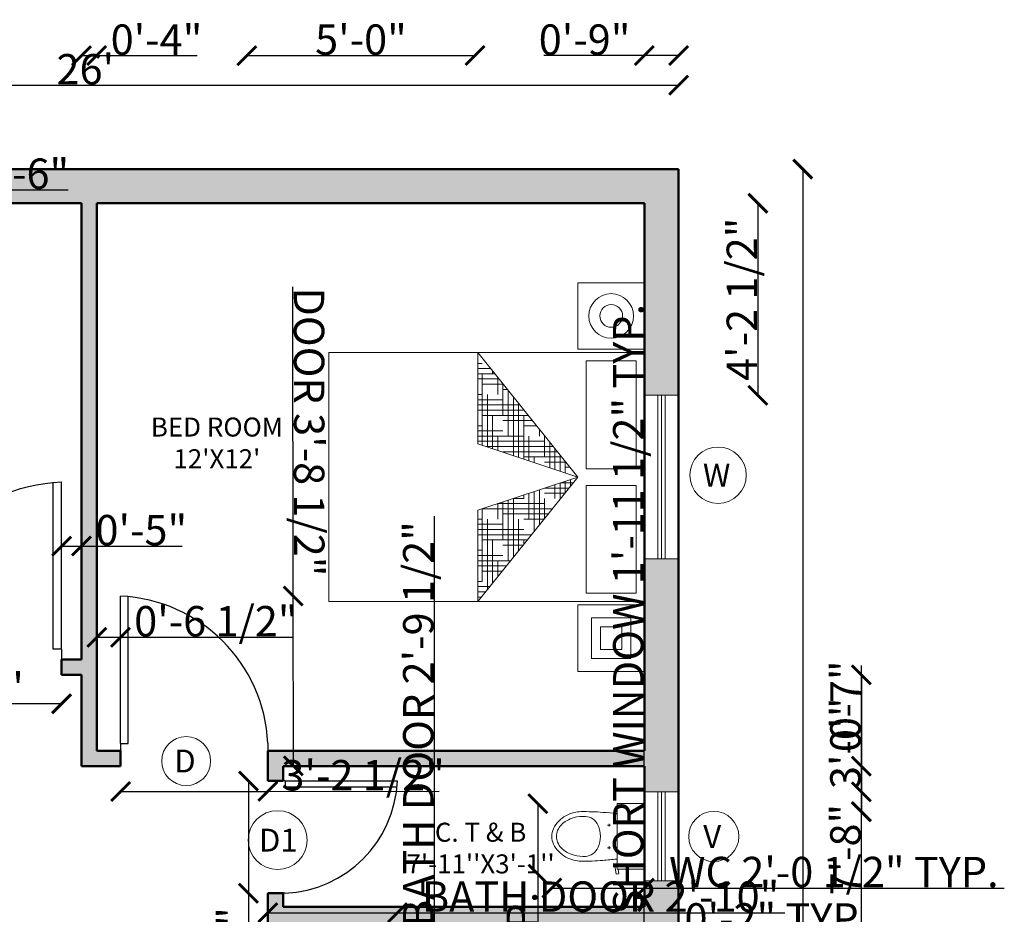
# Model space of a CAD drawing. Units: inches. Extents: x 2169 to 2662, y 1518 to 2151.
# Tile 6 of 6: x 2403 to 2662, y 1916 to 2151. Entities that reach past the tile are written whole.
import ezdxf

# ---------------------------------------------------------------- set-up
doc = ezdxf.new("R2010")
doc.units = ezdxf.units.IN
for name, color, linetype, lineweight in [('A-ANNO-DIMS', 2, 'Continuous', 18), ('A-ANNO-SYMB', 7, 'Continuous', 18), ('A-AREA-IDEN', 7, 'Continuous', 18), ('A-FLOR-FIXT', 9, 'Continuous', 18), ('A-FURN', 8, 'Continuous', 18), ('A-WALL-PATT', 30, 'Continuous', 13), ('Doors', 240, 'Continuous', 30), ('Walls', 7, 'Continuous', 50), ('Windows', 160, 'Continuous', 18)]:
    doc.layers.add(name, color=color, linetype=linetype, lineweight=lineweight)
doc.styles.get("Standard").update_dxf_attribs({"font": 'arial.ttf'})
doc.dimstyles.get("Standard").update_dxf_attribs({"dimtxt": 8, "dimasz": 5, "dimexe": 0.18, "dimexo": 0.0625, "dimgap": 0.09, "dimtad": 1, "dimdec": 1, "dimzin": 0, "dimdsep": 46, "dimlunit": 4, "dimtxsty": 'Standard', "dimblk": 'ARCHTICK', "dimcen": 0.09, "dimse1": 1, "dimse2": 1, "dimadec": 0, "dimazin": 0, "dimtfac": 1, "dimtdec": 1, "dimtofl": 0, "dimtmove": 0, "dimatfit": 3, "dimfxl": 1, "dimtolj": 1, "dimtzin": 0, "dimarcsym": 0})

# ---------------------------------------------------------------- blocks, each defined once
blk = doc.blocks.new('_ArchTick')
at = {"color": 0, "linetype": 'ByBlock', "const_width": 0.15}
blk.add_lwpolyline([(-0.5, -0.5), (0.5, 0.5)], dxfattribs=at)
blk = doc.blocks.new('*D2')
at = {"layer": 'A-ANNO-DIMS', "color": 0, "lineweight": -2, "transparency": 16777216}
blk.add_line((2263.98, 2133.67), (2575.98, 2133.67), dxfattribs=at)
at = {"layer": 'Defpoints', "color": 0, "transparency": 16777216}
for p in [(2575.98, 2133.67), (2263.98, 2111.6), (2575.98, 2111.6)]:
    blk.add_point(p, dxfattribs=at)
at = {"layer": 'A-ANNO-DIMS', "color": 0, "lineweight": -2, "transparency": 16777216, "xscale": 5, "yscale": 5, "zscale": 5, "rotation": 180}
blk.add_blockref('_ArchTick', (2263.98, 2133.67), dxfattribs=at)
at = {"layer": 'A-ANNO-DIMS', "color": 0, "lineweight": -2, "transparency": 16777216, "xscale": 5, "yscale": 5, "zscale": 5}
blk.add_blockref('_ArchTick', (2575.98, 2133.67), dxfattribs=at)
at = {"layer": 'A-ANNO-DIMS', "color": 0, "transparency": 16777216, "insert": (2419.98, 2137.85), "char_height": 8, "attachment_point": 5}
blk.add_mtext("\\A1;26'", dxfattribs=at)
blk = doc.blocks.new('*D3')
at = {"layer": 'A-ANNO-DIMS', "color": 0, "lineweight": -2, "transparency": 16777216}
blk.add_line((2608.61, 2111.6), (2608.61, 1595.6), dxfattribs=at)
at = {"layer": 'Defpoints', "color": 0, "transparency": 16777216}
for p in [(2575.74, 2111.6), (2575.98, 1595.6), (2608.61, 1595.6)]:
    blk.add_point(p, dxfattribs=at)
at = {"layer": 'A-ANNO-DIMS', "color": 0, "lineweight": -2, "transparency": 16777216, "xscale": 5, "yscale": 5, "zscale": 5}
for p, rotation in [((2608.61, 2111.6), 90), ((2608.61, 1595.6), 270)]:
    blk.add_blockref('_ArchTick', p, dxfattribs=dict(at, rotation=rotation))
at = {"layer": 'A-ANNO-DIMS', "color": 0, "transparency": 16777216, "insert": (2604.43, 1853.6), "char_height": 8, "attachment_point": 5, "rotation": 90}
blk.add_mtext("\\A1;43'", dxfattribs=at)
blk = doc.blocks.new('AP0B05')
for p, q in [((35, 100), (35, 880)), ((75, 100), (75, 878.9)), ((35, 100), (35, -20)), ((815, 100), (815, -20))]:
    blk.add_line(p, q)
blk.add_lwpolyline([(35, 100), (75, 100)])
blk.add_arc((-2.4, 62.6), 818.3, 2.6212, 87.3788)
blk = doc.blocks.new('*X16')
at = {"color": 0}
for p, q in [((20.1875, 14.75), (20.1875, 14.7669)), ((20.199, 14.7812), (20.2772, 14.7812)), ((20.25, 14.8125), (20.2772, 14.8125)), ((20.1487, 14.7188), (20.2772, 14.7188)), ((20.1562, 14.625), (20.1562, 14.7281)), ((20.1739, 14.75), (20.2772, 14.75)), ((20.25, 14.3194), (20.25, 14.75)), ((20.0938, 14.375), (20.0938, 14.6504)), ((20.0984, 14.6562), (20.125, 14.6562)), ((20.1236, 14.6875), (20.25, 14.6875)), ((20.125, 14.5), (20.125, 14.6893)), ((20.0625, 14.2573), (20.0625, 14.6116)), ((20.125, 14.5938), (20.2772, 14.5938)), ((20.2188, 14.3091), (20.2188, 14.625)), ((20.25, 14.625), (20.2772, 14.625)), ((19.9979, 14.5312), (20.2772, 14.5312)), ((20.023, 14.5625), (20.2772, 14.5625)), ((20.0312, 14.2469), (20.0312, 14.5727)), ((19.9476, 14.4688), (20.125, 14.4688)), ((19.9727, 14.5), (20.25, 14.5)), ((20, 14.2366), (20, 14.5)), ((20.1875, 14.2987), (20.1875, 14.5)), ((19.9062, 14.375), (19.9062, 14.4174)), ((19.9225, 14.4375), (20, 14.4375)), ((20.125, 14.4062), (20.2772, 14.4062)), ((20.25, 14.4375), (20.2772, 14.4375)), ((19.875, 14.25), (19.875, 14.3785)), ((19.875, 14.3438), (20.2772, 14.3438)), ((19.9688, 14.2262), (19.9688, 14.375)), ((20, 14.375), (20.2772, 14.375)), ((20.1562, 14.2884), (20.1562, 14.375)), ((19.8125, 14.1744), (19.8125, 14.3008)), ((19.8219, 14.3125), (20.2291, 14.3125)), ((19.8438, 14.1848), (19.8438, 14.3397)), ((19.7716, 14.25), (20, 14.25)), ((19.7812, 14.1641), (19.7812, 14.262)), ((19.7967, 14.2812), (20.125, 14.2812)), ((19.9375, 14.2159), (19.9375, 14.25)), ((19.7213, 14.1875), (19.75, 14.1875)), ((19.7465, 14.2188), (19.875, 14.2188)), ((19.75, 14.1537), (19.75, 14.2231)), ((19.7188, 14.0726), (19.7188, 14.1136)), ((19.7018, 14.0938), (19.7786, 14.0938)), ((19.7269, 14.0625), (19.8728, 14.0625)), ((19.75, 14.0338), (19.75, 14.1032)), ((19.7812, 13.9949), (19.7812, 14.0929)), ((19.8125, 14), (19.8125, 14.0825)), ((19.9062, 13.8396), (19.9062, 14.0514)), ((19.752, 14.0312), (19.875, 14.0312)), ((19.875, 13.8784), (19.875, 14)), ((19.9375, 13.8007), (19.9375, 14.0411)), ((19.9688, 13.875), (19.9688, 14.0307)), ((20, 14), (20, 14.0204)), ((20, 14), (20.0614, 14)), ((20.0625, 13.6454), (20.0625, 13.9996)), ((20.0938, 13.625), (20.0938, 13.9893)), ((19.8275, 13.9375), (20.25, 13.9375)), ((19.875, 13.9688), (20.1557, 13.9688)), ((20.125, 13.75), (20.125, 13.9789)), ((20.1562, 13.875), (20.1562, 13.9686)), ((20.25, 13.5), (20.25, 13.9375)), ((19.8526, 13.9062), (20.125, 13.9062)), ((19.8777, 13.875), (20, 13.875)), ((20.0312, 13.6842), (20.0312, 13.875)), ((20.2188, 13.4511), (20.2188, 13.875)), ((20.25, 13.875), (20.2772, 13.875)), ((20, 13.8125), (20.2772, 13.8125)), ((20.125, 13.8438), (20.2772, 13.8438)), ((19.9532, 13.7812), (20.2772, 13.7812)), ((19.9783, 13.75), (20.25, 13.75)), ((20, 13.723), (20, 13.75)), ((20.0035, 13.7188), (20.125, 13.7188)), ((20.1875, 13.49), (20.1875, 13.75)), ((20.125, 13.6562), (20.2772, 13.6562)), ((20.25, 13.6875), (20.2772, 13.6875)), ((20.0789, 13.625), (20.2772, 13.625)), ((20.104, 13.5938), (20.2772, 13.5938)), ((20.1562, 13.5288), (20.1562, 13.625)), ((20.1292, 13.5625), (20.25, 13.5625)), ((20.2046, 13.4688), (20.2772, 13.4688)), ((20.25, 13.5), (20.2772, 13.5)), ((20.2297, 13.4375), (20.2772, 13.4375)), ((20.2549, 13.4062), (20.2772, 13.4062))]:
    blk.add_line(p, q, dxfattribs=at)
blk = doc.blocks.new('MAT-P13')
for p, q in [((-1.17, 0), (-1.17, -0.4)), ((-1.17, 0), (-0.77, 0)), ((-0.77, 0), (-0.77, -0.4)), ((-0.75, 0), (0.75, 0)), ((-0.75, 0), (-0.75, -1.9)), ((0.75, 0), (0.75, -1.9)), ((0.77, 0), (1.17, 0)), ((0.77, 0), (0.77, -0.4)), ((1.17, 0), (1.17, -0.4)), ((-0.7, -0.05), (-0.7, -0.35)), ((-0.7, -0.05), (-0.05, -0.05)), ((-0.05, -0.35), (-0.05, -0.05)), ((0.05, -0.05), (0.7, -0.05)), ((0.05, -0.35), (0.05, -0.05)), ((0.7, -0.05), (0.7, -0.35)), ((-0.7, -0.35), (-0.05, -0.35)), ((0.05, -0.35), (0.7, -0.35)), ((-1.17, -0.4), (-0.77, -0.4)), ((-0.75, -1.0034), (0, -0.4)), ((0, -0.4), (-0.75, -1.0034)), ((0, -0.4), (-0.2, -1.0034)), ((0, -0.4), (0.2, -1.0034)), ((0, -0.4), (0.75, -1.0034)), ((0.77, -0.4), (1.17, -0.4)), ((-0.75, -1.0034), (-0.2, -1.0034)), ((0.2, -1.0034), (0.75, -1.0034)), ((0.75, -1.9), (-0.75, -1.9))]:
    blk.add_line(p, q)
for points in [[(0.8468, -0.0814), (1.0932, -0.0814), (1.0932, -0.3186), (0.8468, -0.3186)], [(0.9015, -0.1361), (1.0385, -0.1361), (1.0385, -0.2639), (0.9015, -0.2639)]]:
    blk.add_lwpolyline(points, close=True)
for radius in [0.1342, 0.0686]:
    blk.add_circle((-0.97, -0.2), radius)
at = {"xscale": -1, "rotation": 90}
blk.add_blockref('*X16', (14.1285, 19.2738), dxfattribs=at)
blk = doc.blocks.new('toilet-1')
at = {"color": 0, "linetype": 'ByBlock'}
for p, q in [((-0.23, -0.02), (-0.23, -0.2116)), ((0.23, -0.02), (-0.23, -0.02)), ((0.23, -0.02), (0.23, -0.2116)), ((0.2633, -0.1997), (0.23, -0.2044)), ((0.266, -0.2187), (0.2633, -0.1997)), ((-0.23, -0.2116), (0.23, -0.2116)), ((-0.0889, -0.2683), (-0.0697, -0.2683)), ((-0.0793, -0.2587), (-0.0793, -0.2778)), ((0.0889, -0.2683), (0.0698, -0.2683)), ((0.0794, -0.2587), (0.0794, -0.2778)), ((0.1917, -0.2144), (0.2206, -0.225)), ((0.2206, -0.225), (0.266, -0.2187)), ((0, -0.6382), (0, -0.6382))]:
    blk.add_line(p, q, dxfattribs=at)
for centre, radius, start, end in [((3.5272, -0.6239), 3.7093, 173.69251, 175.15926), ((-3.527, -0.624), 3.7093, 4.84131, 6.31706), ((1.7368, -0.4519), 1.9109, 175.76982, 180.37578), ((-0.0312, -0.4465), 0.1114, 113.89968, 145.1485), ((0, -0.5169), 0.1884, 66.09393, 113.90607), ((0.0312, -0.4465), 0.1114, 34.8515, 66.10032), ((-1.7366, -0.4519), 1.9109, 359.62422, 4.23018), ((-0.0408, -0.4398), 0.0996, 145.14967, 175.88096), ((0.0409, -0.4398), 0.0996, 4.11904, 34.85033), ((0.0353, -0.463), 0.2093, 180.37466, 194.33753), ((0.0981, -0.4497), 0.2389, 175.88621, 195.59308), ((-0.098, -0.4497), 0.2389, 344.40692, 4.11379), ((-0.0351, -0.463), 0.2093, 345.6614, 359.62427), ((0.055, -0.458), 0.2297, 194.33532, 209.62204), ((0.0961, -0.4503), 0.2369, 195.59686, 209.37705), ((-0.096, -0.4503), 0.2369, 330.62295, 344.40314), ((-0.0548, -0.458), 0.2297, 330.37879, 345.66551), ((0.0647, -0.4524), 0.2409, 209.62726, 224.54888), ((0.0232, -0.4913), 0.1532, 209.38715, 226.54376), ((0.0178, -0.4986), 0.1751, 224.55199, 245.714), ((0.0152, -0.4997), 0.1416, 226.55015, 246.55272), ((-0.0151, -0.4997), 0.1416, 293.44728, 313.44985), ((-0.0176, -0.4986), 0.1751, 294.28649, 315.4485), ((-0.0231, -0.4913), 0.1532, 313.45624, 330.61285), ((-0.0645, -0.4524), 0.2409, 315.45042, 330.37204), ((0.0004, -0.538), 0.132, 245.58449, 269.87817), ((0, -0.5347), 0.1034, 246.54933, 270.0042), ((0, -0.5347), 0.1034, 269.9958, 293.45067), ((-0.0002, -0.538), 0.132, 270.12162, 294.4153)]:
    blk.add_arc(centre, radius, start, end, dxfattribs=at)
blk = doc.blocks.new('GLAZING-43IN')
for p, q in [((-21.5, 1), (21.5, 1)), ((-21.5, 0), (21.5, 0)), ((-21.5, -1), (21.5, -1))]:
    blk.add_line(p, q)
blk = doc.blocks.new('GLAZING-SHORT')
for p, q in [((-1, -11.72), (-1, 11.72)), ((0, -11.72), (0, 11.72)), ((1, -11.72), (1, 11.72))]:
    blk.add_line(p, q)
blk = doc.blocks.new('OPENING-TAG-W')
blk.add_circle((0, 0), 7.42)
blk.add_text('W', height=6).set_placement((-3.96, -3))
blk = doc.blocks.new('OPENING-TAG-D')
blk.add_circle((0, 0), 6.43)
blk.add_text('D', height=6).set_placement((-3.13, -3))
blk = doc.blocks.new('OPENING-TAG-V')
blk.add_circle((0, 0), 6.61)
blk.add_text('V', height=6).set_placement((-2.78, -3))
blk = doc.blocks.new('OPENING-TAG-D1')
blk.add_circle((0, 0), 7.74)
blk.add_text('D1', height=6).set_placement((-4.91, -3.01))
blk = doc.blocks.new('*D27')
at = {"layer": 'A-ANNO-DIMS', "color": 0, "lineweight": -2, "transparency": 16777216}
for p, q in [((2566.96, 1906.83), (2566.96, 2079.95)), ((2566.96, 1883.38), (2566.96, 1906.83))]:
    blk.add_line(p, q, dxfattribs=at)
at = {"layer": 'Defpoints', "color": 0, "transparency": 16777216}
for p in [(2566.96, 1906.83), (2570.48, 1906.83), (2570.48, 1883.38)]:
    blk.add_point(p, dxfattribs=at)
at = {"layer": 'A-ANNO-DIMS', "color": 0, "lineweight": -2, "transparency": 16777216, "xscale": 5, "yscale": 5, "zscale": 5}
for p, rotation in [((2566.96, 1906.83), 90), ((2566.96, 1883.38), 270)]:
    blk.add_blockref('_ArchTick', p, dxfattribs=dict(at, rotation=rotation))
at = {"layer": 'A-ANNO-DIMS', "color": 0, "transparency": 16777216, "insert": (2562.73, 1995.89), "char_height": 8, "attachment_point": 5, "rotation": 90}
blk.add_mtext('\\A1;SHORT WINDOW 1\'-11 1/2" TYP.', dxfattribs=at)
blk = doc.blocks.new('*D28')
at = {"layer": 'A-ANNO-DIMS', "color": 0, "lineweight": -2, "transparency": 16777216}
for p, q in [((2570.48, 1910.34), (2572.48, 1910.34)), ((2572.48, 1910.34), (2626.42, 1910.34))]:
    blk.add_line(p, q, dxfattribs=at)
at = {"layer": 'Defpoints', "color": 0, "transparency": 16777216}
for p in [(2572.48, 1910.34), (2570.48, 1906.83), (2572.48, 1906.83)]:
    blk.add_point(p, dxfattribs=at)
at = {"layer": 'A-ANNO-DIMS', "color": 0, "lineweight": -2, "transparency": 16777216, "xscale": 5, "yscale": 5, "zscale": 5, "rotation": 180}
blk.add_blockref('_ArchTick', (2570.48, 1910.34), dxfattribs=at)
at = {"layer": 'A-ANNO-DIMS', "color": 0, "lineweight": -2, "transparency": 16777216, "xscale": 5, "yscale": 5, "zscale": 5}
blk.add_blockref('_ArchTick', (2572.48, 1910.34), dxfattribs=at)
at = {"layer": 'A-ANNO-DIMS', "color": 0, "transparency": 16777216, "insert": (2601.95, 1914.52), "char_height": 8, "attachment_point": 5}
blk.add_mtext('\\A1;0\'-2" TYP.', dxfattribs=at)
blk = doc.blocks.new('*D29')
at = {"layer": 'A-ANNO-DIMS', "color": 0, "lineweight": -2, "transparency": 16777216}
for p, q in [((2474.64, 1999.32), (2474.57, 2080.64)), ((2474.68, 1954.64), (2474.64, 1999.32))]:
    blk.add_line(p, q, dxfattribs=at)
at = {"layer": 'Defpoints', "color": 0, "transparency": 16777216}
for p in [(2467.94, 1999.31), (2474.64, 1999.32), (2467.98, 1954.64)]:
    blk.add_point(p, dxfattribs=at)
at = {"layer": 'A-ANNO-DIMS', "color": 0, "lineweight": -2, "transparency": 16777216, "xscale": 5, "yscale": 5, "zscale": 5}
for p, rotation in [((2474.64, 1999.32), 90.0482216414707), ((2474.68, 1954.64), 270.0482216414707)]:
    blk.add_blockref('_ArchTick', p, dxfattribs=dict(at, rotation=rotation))
at = {"layer": 'A-ANNO-DIMS', "color": 0, "transparency": 16777216, "insert": (2478.83, 2042.48), "char_height": 8, "attachment_point": 5, "rotation": 270.0482}
blk.add_mtext('\\A1;DOOR 3\'-8 1/2"', dxfattribs=at)
blk = doc.blocks.new('*D30')
at = {"layer": 'A-ANNO-DIMS', "color": 0, "lineweight": -2, "transparency": 16777216}
for p, q in [((2429.26, 1947.9), (2467.98, 1947.94)), ((2467.98, 1947.94), (2513.06, 1947.97))]:
    blk.add_line(p, q, dxfattribs=at)
at = {"layer": 'Defpoints', "color": 0, "transparency": 16777216}
for p in [(2467.98, 1954.64), (2429.26, 1954.6), (2467.98, 1947.94)]:
    blk.add_point(p, dxfattribs=at)
at = {"layer": 'A-ANNO-DIMS', "color": 0, "lineweight": -2, "transparency": 16777216, "xscale": 5, "yscale": 5, "zscale": 5}
for p, rotation in [((2429.26, 1947.9), 180.0482216414703), ((2467.98, 1947.94), 0.0482216414702963)]:
    blk.add_blockref('_ArchTick', p, dxfattribs=dict(at, rotation=rotation))
at = {"layer": 'A-ANNO-DIMS', "color": 0, "transparency": 16777216, "insert": (2493.02, 1952.19), "char_height": 8, "attachment_point": 5, "rotation": 0.0482}
blk.add_mtext('\\A1;3\'-2 1/2"', dxfattribs=at)
blk = doc.blocks.new('*D32')
at = {"layer": 'A-ANNO-DIMS', "color": 0, "lineweight": -2, "transparency": 16777216}
blk.add_line((2413.75, 1970.99), (2369.77, 1970.99), dxfattribs=at)
at = {"layer": 'Defpoints', "color": 0, "transparency": 16777216}
for p in [(2369.77, 1978.6), (2413.75, 1978.6), (2369.77, 1970.99)]:
    blk.add_point(p, dxfattribs=at)
at = {"layer": 'A-ANNO-DIMS', "color": 0, "lineweight": -2, "transparency": 16777216, "xscale": 5, "yscale": 5, "zscale": 5, "rotation": 180}
blk.add_blockref('_ArchTick', (2369.77, 1970.99), dxfattribs=at)
at = {"layer": 'A-ANNO-DIMS', "color": 0, "lineweight": -2, "transparency": 16777216, "xscale": 5, "yscale": 5, "zscale": 5}
blk.add_blockref('_ArchTick', (2413.75, 1970.99), dxfattribs=at)
at = {"layer": 'A-ANNO-DIMS', "color": 0, "transparency": 16777216, "insert": (2391.76, 1975.17), "char_height": 8, "attachment_point": 5}
blk.add_mtext('\\A1;3\'-8"', dxfattribs=at)
blk = doc.blocks.new('*D33')
at = {"layer": 'A-ANNO-DIMS', "color": 0, "lineweight": -2, "transparency": 16777216}
for p, q in [((2467.98, 1916.03), (2502.05, 1916.03)), ((2502.05, 1916.03), (2603.9, 1916.03))]:
    blk.add_line(p, q, dxfattribs=at)
at = {"layer": 'Defpoints', "color": 0, "transparency": 16777216}
for p in [(2467.98, 1921.14), (2502.05, 1921.14), (2502.05, 1916.03)]:
    blk.add_point(p, dxfattribs=at)
at = {"layer": 'A-ANNO-DIMS', "color": 0, "lineweight": -2, "transparency": 16777216, "xscale": 5, "yscale": 5, "zscale": 5, "rotation": 180}
blk.add_blockref('_ArchTick', (2467.98, 1916.03), dxfattribs=at)
at = {"layer": 'A-ANNO-DIMS', "color": 0, "lineweight": -2, "transparency": 16777216, "xscale": 5, "yscale": 5, "zscale": 5}
blk.add_blockref('_ArchTick', (2502.05, 1916.03), dxfattribs=at)
at = {"layer": 'A-ANNO-DIMS', "color": 0, "transparency": 16777216, "insert": (2555.47, 1920.26), "char_height": 8, "attachment_point": 5}
blk.add_mtext('\\A1;BATH DOOR 2\'-10"', dxfattribs=at)
blk = doc.blocks.new('*D34')
at = {"layer": 'A-ANNO-DIMS', "color": 0, "lineweight": -2, "transparency": 16777216}
for p, q in [((2462.86, 1950.67), (2462.86, 1921.14)), ((2462.86, 1921.14), (2462.86, 1875.92))]:
    blk.add_line(p, q, dxfattribs=at)
at = {"layer": 'Defpoints', "color": 0, "transparency": 16777216}
for p in [(2467.98, 1950.67), (2462.86, 1921.14), (2467.98, 1921.14)]:
    blk.add_point(p, dxfattribs=at)
at = {"layer": 'A-ANNO-DIMS', "color": 0, "lineweight": -2, "transparency": 16777216, "xscale": 5, "yscale": 5, "zscale": 5}
for p, rotation in [((2462.86, 1950.67), 90), ((2462.86, 1921.14), 270)]:
    blk.add_blockref('_ArchTick', p, dxfattribs=dict(at, rotation=rotation))
at = {"layer": 'A-ANNO-DIMS', "color": 0, "transparency": 16777216, "insert": (2458.64, 1896.03), "char_height": 8, "attachment_point": 5, "rotation": 90}
blk.add_mtext('\\A1;2\'-5 1/2"', dxfattribs=at)
blk = doc.blocks.new('*D39')
at = {"layer": 'A-ANNO-DIMS', "color": 0, "lineweight": -2, "transparency": 16777216}
for p, q in [((2511.76, 1906), (2511.76, 2020.27)), ((2511.76, 1872.6), (2511.76, 1906))]:
    blk.add_line(p, q, dxfattribs=at)
at = {"layer": 'Defpoints', "color": 0, "transparency": 16777216}
for p in [(2506.75, 1906), (2511.76, 1906), (2506.75, 1872.6)]:
    blk.add_point(p, dxfattribs=at)
at = {"layer": 'A-ANNO-DIMS', "color": 0, "lineweight": -2, "transparency": 16777216, "xscale": 5, "yscale": 5, "zscale": 5}
for p, rotation in [((2511.76, 1906), 90), ((2511.76, 1872.6), 270)]:
    blk.add_blockref('_ArchTick', p, dxfattribs=dict(at, rotation=rotation))
at = {"layer": 'A-ANNO-DIMS', "color": 0, "transparency": 16777216, "insert": (2507.53, 1965.63), "char_height": 8, "attachment_point": 5, "rotation": 90}
blk.add_mtext('\\A1;BATH DOOR 2\'-9 1/2"', dxfattribs=at)
blk = doc.blocks.new('*D49')
at = {"layer": 'A-ANNO-DIMS', "color": 0, "lineweight": -2, "transparency": 16777216}
for p, q in [((2542.64, 1922.5), (2566.98, 1922.5)), ((2566.98, 1922.5), (2661.61, 1922.5))]:
    blk.add_line(p, q, dxfattribs=at)
at = {"layer": 'Defpoints', "color": 0, "transparency": 16777216}
for p in [(2542.64, 1926.15), (2566.98, 1926.15), (2566.98, 1922.5)]:
    blk.add_point(p, dxfattribs=at)
at = {"layer": 'A-ANNO-DIMS', "color": 0, "lineweight": -2, "transparency": 16777216, "xscale": 5, "yscale": 5, "zscale": 5, "rotation": 180}
blk.add_blockref('_ArchTick', (2542.64, 1922.5), dxfattribs=at)
at = {"layer": 'A-ANNO-DIMS', "color": 0, "lineweight": -2, "transparency": 16777216, "xscale": 5, "yscale": 5, "zscale": 5}
blk.add_blockref('_ArchTick', (2566.98, 1922.5), dxfattribs=at)
at = {"layer": 'A-ANNO-DIMS', "color": 0, "transparency": 16777216, "insert": (2616.79, 1926.72), "char_height": 8, "attachment_point": 5}
blk.add_mtext('\\A1;WC 2\'-0 1/2" TYP.', dxfattribs=at)
blk = doc.blocks.new('*D50')
at = {"layer": 'A-ANNO-DIMS', "color": 0, "lineweight": -2, "transparency": 16777216}
for p, q in [((2538.99, 1944.71), (2538.99, 1926.15)), ((2538.99, 1926.15), (2538.99, 1854.31))]:
    blk.add_line(p, q, dxfattribs=at)
at = {"layer": 'Defpoints', "color": 0, "transparency": 16777216}
for p in [(2542.64, 1944.71), (2538.99, 1926.15), (2542.64, 1926.15)]:
    blk.add_point(p, dxfattribs=at)
at = {"layer": 'A-ANNO-DIMS', "color": 0, "lineweight": -2, "transparency": 16777216, "xscale": 5, "yscale": 5, "zscale": 5}
for p, rotation in [((2538.99, 1944.71), 90), ((2538.99, 1926.15), 270)]:
    blk.add_blockref('_ArchTick', p, dxfattribs=dict(at, rotation=rotation))
at = {"layer": 'A-ANNO-DIMS', "color": 0, "transparency": 16777216, "insert": (2534.77, 1887.73), "char_height": 8, "attachment_point": 5, "rotation": 90}
blk.add_mtext('\\A1;1\'-6 1/2" TYP.', dxfattribs=at)
blk = doc.blocks.new('*D53')
at = {"layer": 'A-ANNO-DIMS', "color": 0, "lineweight": -2, "transparency": 16777216}
for p, q in [((2317.71, 2106.14), (2359.84, 2106.14)), ((2359.84, 2106.14), (2415.44, 2106.14))]:
    blk.add_line(p, q, dxfattribs=at)
at = {"layer": 'Defpoints', "color": 0, "transparency": 16777216}
for p in [(2359.84, 2106.14), (2317.71, 2099.82), (2359.84, 2099.82)]:
    blk.add_point(p, dxfattribs=at)
at = {"layer": 'A-ANNO-DIMS', "color": 0, "lineweight": -2, "transparency": 16777216, "xscale": 5, "yscale": 5, "zscale": 5, "rotation": 180}
blk.add_blockref('_ArchTick', (2317.71, 2106.14), dxfattribs=at)
at = {"layer": 'A-ANNO-DIMS', "color": 0, "lineweight": -2, "transparency": 16777216, "xscale": 5, "yscale": 5, "zscale": 5}
blk.add_blockref('_ArchTick', (2359.84, 2106.14), dxfattribs=at)
at = {"layer": 'A-ANNO-DIMS', "color": 0, "transparency": 16777216, "insert": (2390.14, 2110.37), "char_height": 8, "attachment_point": 5}
blk.add_mtext('\\A1;SINK 3\'-6"', dxfattribs=at)
blk = doc.blocks.new('*D55')
at = {"layer": 'A-ANNO-DIMS', "color": 0, "lineweight": -2, "transparency": 16777216}
blk.add_line((2462.45, 2141.45), (2522.45, 2141.45), dxfattribs=at)
at = {"layer": 'Defpoints', "color": 0, "transparency": 16777216}
for p in [(2522.45, 2141.45), (2462.45, 1604.6), (2522.45, 1604.6)]:
    blk.add_point(p, dxfattribs=at)
at = {"layer": 'A-ANNO-DIMS', "color": 0, "lineweight": -2, "transparency": 16777216, "xscale": 5, "yscale": 5, "zscale": 5, "rotation": 180}
blk.add_blockref('_ArchTick', (2462.45, 2141.45), dxfattribs=at)
at = {"layer": 'A-ANNO-DIMS', "color": 0, "lineweight": -2, "transparency": 16777216, "xscale": 5, "yscale": 5, "zscale": 5}
blk.add_blockref('_ArchTick', (2522.45, 2141.45), dxfattribs=at)
at = {"layer": 'A-ANNO-DIMS', "color": 0, "transparency": 16777216, "insert": (2492.45, 2145.63), "char_height": 8, "attachment_point": 5}
blk.add_mtext('\\A1;5\'-0"', dxfattribs=at)
blk = doc.blocks.new('*D63')
at = {"layer": 'A-ANNO-DIMS', "color": 0, "lineweight": -2, "transparency": 16777216}
blk.add_line((2596.83, 2102.6), (2596.83, 2052.1), dxfattribs=at)
at = {"layer": 'Defpoints', "color": 0, "transparency": 16777216}
for p in [(2566.98, 2102.6), (2566.98, 2052.1), (2596.83, 2052.1)]:
    blk.add_point(p, dxfattribs=at)
at = {"layer": 'A-ANNO-DIMS', "color": 0, "lineweight": -2, "transparency": 16777216, "xscale": 5, "yscale": 5, "zscale": 5}
for p, rotation in [((2596.83, 2102.6), 90), ((2596.83, 2052.1), 270)]:
    blk.add_blockref('_ArchTick', p, dxfattribs=dict(at, rotation=rotation))
at = {"layer": 'A-ANNO-DIMS', "color": 0, "transparency": 16777216, "insert": (2592.6, 2077.35), "char_height": 8, "attachment_point": 5, "rotation": 90}
blk.add_mtext('\\A1;4\'-2 1/2"', dxfattribs=at)
blk = doc.blocks.new('*D66')
at = {"layer": 'A-ANNO-DIMS', "color": 0, "lineweight": -2, "transparency": 16777216}
for p, q in [((2566.98, 2141.45), (2540.53, 2141.45)), ((2575.98, 2141.45), (2566.98, 2141.45))]:
    blk.add_line(p, q, dxfattribs=at)
at = {"layer": 'Defpoints', "color": 0, "transparency": 16777216}
for p in [(2566.98, 2141.45), (2575.98, 2111.6), (2566.98, 2102.6)]:
    blk.add_point(p, dxfattribs=at)
at = {"layer": 'A-ANNO-DIMS', "color": 0, "lineweight": -2, "transparency": 16777216, "xscale": 5, "yscale": 5, "zscale": 5, "rotation": 180}
blk.add_blockref('_ArchTick', (2566.98, 2141.45), dxfattribs=at)
at = {"layer": 'A-ANNO-DIMS', "color": 0, "lineweight": -2, "transparency": 16777216, "xscale": 5, "yscale": 5, "zscale": 5}
blk.add_blockref('_ArchTick', (2575.98, 2141.45), dxfattribs=at)
at = {"layer": 'A-ANNO-DIMS', "color": 0, "transparency": 16777216, "insert": (2551.25, 2145.63), "char_height": 8, "attachment_point": 5}
blk.add_mtext('\\A1;0\'-9"', dxfattribs=at)
blk = doc.blocks.new('*D67')
at = {"layer": 'A-ANNO-DIMS', "color": 0, "lineweight": -2, "transparency": 16777216}
for p, q in [((2418.98, 2141.45), (2422.98, 2141.45)), ((2422.98, 2141.45), (2449.42, 2141.45))]:
    blk.add_line(p, q, dxfattribs=at)
at = {"layer": 'Defpoints', "color": 0, "transparency": 16777216}
for p in [(2422.98, 2141.45), (2418.98, 2102.6), (2422.98, 2102.6)]:
    blk.add_point(p, dxfattribs=at)
at = {"layer": 'A-ANNO-DIMS', "color": 0, "lineweight": -2, "transparency": 16777216, "xscale": 5, "yscale": 5, "zscale": 5, "rotation": 180}
blk.add_blockref('_ArchTick', (2418.98, 2141.45), dxfattribs=at)
at = {"layer": 'A-ANNO-DIMS', "color": 0, "lineweight": -2, "transparency": 16777216, "xscale": 5, "yscale": 5, "zscale": 5}
blk.add_blockref('_ArchTick', (2422.98, 2141.45), dxfattribs=at)
at = {"layer": 'A-ANNO-DIMS', "color": 0, "transparency": 16777216, "insert": (2438.7, 2145.63), "char_height": 8, "attachment_point": 5}
blk.add_mtext('\\A1;0\'-4"', dxfattribs=at)
blk = doc.blocks.new('*D72')
at = {"layer": 'A-ANNO-DIMS', "color": 0, "lineweight": -2, "transparency": 16777216}
blk.add_line((2624.02, 1978.6), (2624.02, 1942.6), dxfattribs=at)
at = {"layer": 'Defpoints', "color": 0, "transparency": 16777216}
for p in [(2299.77, 1978.6), (2300.05, 1942.6), (2624.02, 1942.6)]:
    blk.add_point(p, dxfattribs=at)
at = {"layer": 'A-ANNO-DIMS', "color": 0, "lineweight": -2, "transparency": 16777216, "xscale": 5, "yscale": 5, "zscale": 5}
for p, rotation in [((2624.02, 1978.6), 90), ((2624.02, 1942.6), 270)]:
    blk.add_blockref('_ArchTick', p, dxfattribs=dict(at, rotation=rotation))
at = {"layer": 'A-ANNO-DIMS', "color": 0, "transparency": 16777216, "insert": (2619.84, 1960.6), "char_height": 8, "attachment_point": 5, "rotation": 90}
blk.add_mtext('\\A1;3\'-0"', dxfattribs=at)
blk = doc.blocks.new('*D73')
at = {"layer": 'A-ANNO-DIMS', "color": 0, "lineweight": -2, "transparency": 16777216}
blk.add_line((2624.02, 1886.6), (2624.02, 1978.6), dxfattribs=at)
at = {"layer": 'Defpoints', "color": 0, "transparency": 16777216}
for p in [(2369.77, 1978.6), (2624.02, 1978.6), (2370.48, 1886.6)]:
    blk.add_point(p, dxfattribs=at)
at = {"layer": 'A-ANNO-DIMS', "color": 0, "lineweight": -2, "transparency": 16777216, "xscale": 5, "yscale": 5, "zscale": 5}
for p, rotation in [((2624.02, 1978.6), 90), ((2624.02, 1886.6), 270)]:
    blk.add_blockref('_ArchTick', p, dxfattribs=dict(at, rotation=rotation))
at = {"layer": 'A-ANNO-DIMS', "color": 0, "transparency": 16777216, "insert": (2619.84, 1932.6), "char_height": 8, "attachment_point": 5, "rotation": 90}
blk.add_mtext('\\A1;7\'-8"', dxfattribs=at)
blk = doc.blocks.new('*D76')
at = {"layer": 'A-ANNO-DIMS', "color": 0, "lineweight": -2, "transparency": 16777216}
for p, q in [((2624.02, 1954.6), (2624.02, 1981.05)), ((2624.02, 1947.83), (2624.02, 1954.6))]:
    blk.add_line(p, q, dxfattribs=at)
at = {"layer": 'Defpoints', "color": 0, "transparency": 16777216}
for p in [(2566.98, 1954.6), (2624.02, 1954.6), (2566.98, 1947.83)]:
    blk.add_point(p, dxfattribs=at)
at = {"layer": 'A-ANNO-DIMS', "color": 0, "lineweight": -2, "transparency": 16777216, "xscale": 5, "yscale": 5, "zscale": 5}
for p, rotation in [((2624.02, 1954.6), 90), ((2624.02, 1947.83), 270)]:
    blk.add_blockref('_ArchTick', p, dxfattribs=dict(at, rotation=rotation))
at = {"layer": 'A-ANNO-DIMS', "color": 0, "transparency": 16777216, "insert": (2619.84, 1970.33), "char_height": 8, "attachment_point": 5, "rotation": 90}
blk.add_mtext('\\A1;0\'-7"', dxfattribs=at)
blk = doc.blocks.new('*D84')
at = {"layer": 'A-ANNO-DIMS', "color": 0, "lineweight": -2, "transparency": 16777216}
for p, q in [((2422.98, 1988.45), (2429.26, 1988.45)), ((2429.26, 1988.45), (2474.35, 1988.45))]:
    blk.add_line(p, q, dxfattribs=at)
at = {"layer": 'Defpoints', "color": 0, "transparency": 16777216}
for p in [(2429.26, 1988.45), (2422.98, 1958.6), (2429.26, 1958.6)]:
    blk.add_point(p, dxfattribs=at)
at = {"layer": 'A-ANNO-DIMS', "color": 0, "lineweight": -2, "transparency": 16777216, "xscale": 5, "yscale": 5, "zscale": 5, "rotation": 180}
blk.add_blockref('_ArchTick', (2422.98, 1988.45), dxfattribs=at)
at = {"layer": 'A-ANNO-DIMS', "color": 0, "lineweight": -2, "transparency": 16777216, "xscale": 5, "yscale": 5, "zscale": 5}
blk.add_blockref('_ArchTick', (2429.26, 1988.45), dxfattribs=at)
at = {"layer": 'A-ANNO-DIMS', "color": 0, "transparency": 16777216, "insert": (2454.3, 1992.68), "char_height": 8, "attachment_point": 5}
blk.add_mtext('\\A1;0\'-6 1/2"', dxfattribs=at)
blk = doc.blocks.new('*D85')
at = {"layer": 'A-ANNO-DIMS', "color": 0, "lineweight": -2, "transparency": 16777216}
for p, q in [((2413.75, 2012.45), (2418.98, 2012.45)), ((2418.98, 2012.45), (2445.42, 2012.45))]:
    blk.add_line(p, q, dxfattribs=at)
at = {"layer": 'Defpoints', "color": 0, "transparency": 16777216}
for p in [(2418.98, 2012.45), (2413.75, 1982.6), (2418.98, 1982.6)]:
    blk.add_point(p, dxfattribs=at)
at = {"layer": 'A-ANNO-DIMS', "color": 0, "lineweight": -2, "transparency": 16777216, "xscale": 5, "yscale": 5, "zscale": 5, "rotation": 180}
blk.add_blockref('_ArchTick', (2413.75, 2012.45), dxfattribs=at)
at = {"layer": 'A-ANNO-DIMS', "color": 0, "lineweight": -2, "transparency": 16777216, "xscale": 5, "yscale": 5, "zscale": 5}
blk.add_blockref('_ArchTick', (2418.98, 2012.45), dxfattribs=at)
at = {"layer": 'A-ANNO-DIMS', "color": 0, "transparency": 16777216, "insert": (2434.7, 2016.63), "char_height": 8, "attachment_point": 5}
blk.add_mtext('\\A1;0\'-5"', dxfattribs=at)

msp = doc.modelspace()

# ---------------------------------------------------------------- hatches: boundary and pattern name
at = {"layer": 'A-WALL-PATT', "transparency": 33554585}
h = msp.add_hatch(color=256, dxfattribs=at)
h.dxf.hatch_style = 1
h.paths.add_polyline_path([(2575.98, 2111.6), (2263.98, 2111.6), (2263.98, 2066.68), (2272.98, 2066.68), (2272.98, 2102.6), (2418.98, 2102.6), (2418.98, 1982.6), (2413.75, 1982.6), (2413.75, 1978.6), (2418.98, 1978.6), (2418.98, 1954.6), (2429.26, 1954.6), (2429.26, 1958.6), (2422.98, 1958.6), (2422.98, 2102.6), (2566.98, 2102.6), (2566.98, 2052.1), (2575.98, 2052.1)])
h.paths.add_polyline_path([(2575.98, 2009.1), (2566.98, 2009.1), (2566.98, 1997.84), (2566.98, 1958.6), (2467.98, 1958.6), (2467.98, 1950.67), (2471.98, 1950.67), (2471.98, 1954.6), (2566.98, 1954.6), (2566.98, 1947.83), (2575.98, 1947.83)])
h.paths.add_polyline_path([(2272.98, 2023.68), (2263.98, 2023.68), (2263.98, 1944.7), (2272.98, 1944.7), (2272.98, 1978.6), (2369.77, 1978.6), (2369.77, 1982.6), (2272.98, 1982.6)])
h.paths.add_polyline_path([(2272.98, 1882.6), (2370.48, 1882.6), (2370.48, 1886.6), (2272.98, 1886.6), (2272.98, 1921.26), (2263.98, 1921.26), (2263.98, 1841.55), (2272.98, 1841.55)])
h.paths.add_polyline_path([(2272.98, 1798.55), (2263.98, 1798.55), (2263.98, 1689.49), (2272.98, 1689.49)])
h.paths.add_polyline_path([(2272.98, 1646.49), (2263.98, 1646.49), (2263.98, 1595.6), (2281.85, 1595.6), (2281.85, 1604.6), (2272.98, 1604.6)])
h.paths.add_polyline_path([(2342.72, 1600.02), (2342.72, 1604.6), (2324.85, 1604.6), (2324.85, 1595.6), (2342.72, 1595.6)])
h.paths.add_polyline_path([(2462.45, 1604.6), (2408.92, 1604.6), (2408.92, 1595.6), (2462.45, 1595.6)])
h.paths.add_polyline_path([(2422.98, 1689.75), (2418.98, 1689.75), (2418.98, 1604.6), (2422.98, 1604.6)])
h.paths.add_polyline_path([(2575.98, 1655.1), (2566.98, 1655.1), (2566.98, 1643.84), (2566.98, 1604.6), (2522.45, 1604.6), (2522.45, 1595.6), (2575.98, 1595.6)])
h.paths.add_polyline_path([(2575.98, 1791.1), (2566.98, 1791.1), (2566.98, 1752.6), (2422.98, 1752.6), (2422.98, 1816.31), (2418.98, 1816.31), (2418.98, 1729.93), (2422.98, 1729.93), (2422.98, 1748.6), (2566.98, 1748.6), (2566.98, 1698.1), (2575.98, 1698.1)])
h.paths.add_polyline_path([(2575.98, 1883.38), (2566.98, 1883.38), (2566.98, 1876.6), (2506.75, 1876.6), (2506.75, 1872.6), (2566.98, 1872.6), (2566.98, 1834.1), (2575.98, 1834.1)])
h.paths.add_polyline_path([(2477.81, 1876.6), (2471.98, 1876.6), (2471.98, 1913.6), (2566.98, 1913.6), (2566.98, 1906.83), (2575.98, 1906.83), (2575.98, 1924.38), (2566.98, 1924.38), (2566.98, 1917.6), (2471.98, 1917.6), (2471.98, 1921.14), (2467.98, 1921.14), (2467.98, 1876.6), (2418.98, 1876.6), (2418.98, 1855.49), (2422.98, 1855.49), (2422.98, 1872.6), (2477.81, 1872.6)])

# ---------------------------------------------------------------- linework, layer by layer
at = {"layer": 'Walls'}
for p, q in [((2263.98, 2111.6), (2575.98, 2111.6)), ((2575.98, 2111.6), (2575.98, 1595.6)), ((2272.98, 2102.6), (2418.98, 2102.6)), ((2418.98, 2102.6), (2418.98, 1982.6)), ((2422.98, 2102.6), (2422.98, 1958.6)), ((2422.98, 2102.6), (2566.98, 2102.6)), ((2566.98, 2102.6), (2566.98, 1958.6)), ((2413.75, 1978.6), (2413.75, 1982.6)), ((2413.75, 1982.6), (2418.98, 1982.6)), ((2413.75, 1978.6), (2418.98, 1978.6)), ((2418.98, 1978.6), (2418.98, 1954.6)), ((2422.98, 1958.6), (2429.26, 1958.6)), ((2429.26, 1954.6), (2429.26, 1958.6)), ((2467.98, 1958.6), (2467.98, 1950.67)), ((2467.98, 1958.6), (2566.98, 1958.6)), ((2418.98, 1954.6), (2429.26, 1954.6)), ((2471.98, 1954.6), (2471.98, 1950.67)), ((2471.98, 1954.6), (2566.98, 1954.6)), ((2566.98, 1954.6), (2566.98, 1917.6)), ((2467.98, 1950.67), (2471.98, 1950.67)), ((2467.98, 1921.14), (2471.98, 1921.14)), ((2467.98, 1921.14), (2467.98, 1876.6)), ((2471.98, 1921.14), (2471.98, 1917.6)), ((2471.98, 1917.6), (2566.98, 1917.6))]:
    msp.add_line(p, q, dxfattribs=at)
at = {"layer": 'Windows'}
for points in [[(2566.98, 2009.1), (2566.98, 2052.1), (2575.98, 2052.1), (2575.98, 2009.1)], [(2566.98, 1924.38), (2566.98, 1947.83), (2575.98, 1947.83), (2575.98, 1924.38)]]:
    msp.add_lwpolyline(points, close=True, dxfattribs=at)

# ---------------------------------------------------------------- block references
at = {"layer": 'A-ANNO-SYMB'}
for name, p in [('OPENING-TAG-W', (2586.34, 2031.08)), ('OPENING-TAG-D', (2446.5, 1955.91)), ('OPENING-TAG-D1', (2470.55, 1935.12)), ('OPENING-TAG-V', (2585.23, 1936.07))]:
    msp.add_blockref(name, p, dxfattribs=at)
at = {"layer": 'A-FLOR-FIXT', "xscale": 37.43636210933806, "yscale": 37.43636210933806, "zscale": 37.43636210933806, "rotation": 270}
msp.add_blockref('toilet-1', (2567.72, 1936.1), dxfattribs=at)
at = {"layer": 'A-FURN', "xscale": 43.68114050857687, "yscale": 43.68114050857687, "zscale": 43.68114050857687, "rotation": 270}
msp.add_blockref('MAT-P13', (2566.98, 2030.6), dxfattribs=at)
at = {"layer": 'Doors', "xscale": -0.0563843061810126, "yscale": 0.0563843061810126, "zscale": 0.0563843061810126}
msp.add_blockref('AP0B05', (2415.72, 1979.73), dxfattribs=at)
at = {"layer": 'Doors'}
for p, xscale, yscale, zscale, rotation in [((2427.52, 1955.6), 0.0496374164220387, 0.0496374164220387, 0.0496374164220387, 0.048221641470343), ((2468.73, 1951.99), 0.0378587118445724, 0.0378587118445724, 0.0378587118445724, 269.9999999999979)]:
    msp.add_blockref('AP0B05', p, dxfattribs=dict(at, xscale=xscale, yscale=yscale, zscale=zscale, rotation=rotation))
at = {"layer": 'Windows', "rotation": 89.99999999999991}
msp.add_blockref('GLAZING-43IN', (2571.48, 2030.6), dxfattribs=at)
at = {"layer": 'Windows'}
msp.add_blockref('GLAZING-SHORT', (2571.48, 1936.1), dxfattribs=at)

# ---------------------------------------------------------------- texts
at = {"layer": 'A-AREA-IDEN', "char_height": 5, "attachment_point": 1}
for s, insert in [("\\pxqc;BED ROOM\\P12'X12'", (2422.98, 2046.25)), ("\\pxqc;C. T & B\\P7'-11''X3'-1''", (2492.32, 1939.69))]:
    msp.add_mtext_dynamic_manual_height_columns(s, width=63.1797, gutter_width=12.5, heights=[0], dxfattribs=dict(at, insert=insert))

# ---------------------------------------------------------------- dimensions: what is measured, and where the dimension line sits
at = {"layer": 'A-ANNO-DIMS'}
for base, p1, p2, override, picture, middle in [((2422.98, 2141.45), (2418.98, 2102.6), (2422.98, 2102.6), {"dimdec": 1, "dimlfac": 1, "dimrnd": 0, "dimzin": 1, "dimdsep": 46, "dimlunit": 4, "dimfrac": 2}, '*D67', (2438.7, 2145.63)), ((2522.45, 2141.45), (2462.45, 1604.6), (2522.45, 1604.6), {"dimdec": 1, "dimlfac": 1, "dimrnd": 0, "dimzin": 1, "dimdsep": 46, "dimlunit": 4, "dimfrac": 2}, '*D55', (2492.45, 2145.63)), ((2566.98, 2141.45), (2575.98, 2111.6), (2566.98, 2102.6), {"dimdec": 1, "dimlfac": 1, "dimrnd": 0, "dimzin": 1, "dimdsep": 46, "dimlunit": 4, "dimfrac": 2}, '*D66', (2551.25, 2145.63)), ((2575.98, 2133.67), (2263.98, 2111.6), (2575.98, 2111.6), {"dimclrd": 0, "dimclre": 0, "dimclrt": 0}, '*D2', (2419.98, 2137.85)), ((2429.26, 1988.45), (2422.98, 1958.6), (2429.26, 1958.6), {"dimdec": 1, "dimlfac": 1, "dimrnd": 0, "dimzin": 1, "dimdsep": 46, "dimlunit": 4, "dimfrac": 2}, '*D84', (2454.3, 1992.68))]:
    dim = msp.add_linear_dim(base=base, p1=p1, p2=p2, dimstyle='Standard', override=override, dxfattribs=at)
    dim.commit()
    dim.dimension.update_dxf_attribs({"geometry": picture, "text_midpoint": middle})
for base, p1, p2, text, picture, middle in [((2359.84, 2106.14), (2317.71, 2099.82), (2359.84, 2099.82), 'SINK <>', '*D53', (2390.14, 2110.37)), ((2566.98, 1922.5), (2542.64, 1926.15), (2566.98, 1926.15), 'WC <> TYP.', '*D49', (2616.79, 1926.72)), ((2502.05, 1916.03), (2467.98, 1921.14), (2502.05, 1921.14), 'BATH DOOR <>', '*D33', (2555.47, 1920.26)), ((2572.48, 1910.34), (2570.48, 1906.83), (2572.48, 1906.83), '<> TYP.', '*D28', (2601.95, 1914.52))]:
    dim = msp.add_linear_dim(base=base, p1=p1, p2=p2, text=text, dimstyle='Standard', override={"dimdec": 1, "dimlfac": 1, "dimrnd": 0, "dimzin": 1, "dimdsep": 46, "dimlunit": 4, "dimfrac": 2}, dxfattribs=at)
    dim.commit()
    dim.dimension.update_dxf_attribs({"geometry": picture, "text_midpoint": middle})
for base, p1, p2, angle, override, picture, middle in [((2608.61, 1595.6), (2575.74, 2111.6), (2575.98, 1595.6), 90, {"dimclrd": 0, "dimclre": 0, "dimclrt": 0}, '*D3', (2604.43, 1853.6)), ((2596.83, 2052.1), (2566.98, 2102.6), (2566.98, 2052.1), 270, {"dimdec": 1, "dimlfac": 1, "dimrnd": 0, "dimzin": 1, "dimdsep": 46, "dimlunit": 4, "dimfrac": 2}, '*D63', (2592.6, 2077.35)), ((2418.98, 2012.45), (2413.75, 1982.6), (2418.98, 1982.6), 0, {"dimdec": 1, "dimlfac": 1, "dimrnd": 0, "dimzin": 1, "dimdsep": 46, "dimlunit": 4, "dimfrac": 2}, '*D85', (2434.7, 2016.63)), ((2624.02, 1942.6), (2299.77, 1978.6), (2300.05, 1942.6), 90, {"dimdec": 1, "dimlfac": 1, "dimrnd": 0, "dimzin": 1, "dimdsep": 46, "dimlunit": 4, "dimfrac": 2}, '*D72', (2619.84, 1960.6)), ((2624.02, 1978.6), (2370.48, 1886.6), (2369.77, 1978.6), 90, {"dimdec": 1, "dimlfac": 1, "dimrnd": 0, "dimzin": 1, "dimdsep": 46, "dimlunit": 4, "dimfrac": 2}, '*D73', (2619.84, 1932.6)), ((2624.02, 1954.6), (2566.98, 1947.83), (2566.98, 1954.6), 90, {"dimdec": 1, "dimlfac": 1, "dimrnd": 0, "dimzin": 1, "dimdsep": 46, "dimlunit": 4, "dimfrac": 2}, '*D76', (2619.84, 1970.33)), ((2369.77, 1970.99), (2413.75, 1978.6), (2369.77, 1978.6), 180, {"dimdec": 1, "dimlfac": 1, "dimrnd": 0, "dimzin": 1, "dimdsep": 46, "dimlunit": 4, "dimfrac": 2}, '*D32', (2391.76, 1975.17)), ((2467.98, 1947.94), (2429.26, 1954.6), (2467.98, 1954.64), 0.0482, {"dimdec": 1, "dimlfac": 1, "dimrnd": 0, "dimzin": 1, "dimdsep": 46, "dimlunit": 4, "dimfrac": 2}, '*D30', (2493.02, 1952.19)), ((2462.86, 1921.14), (2467.98, 1950.67), (2467.98, 1921.14), 270, {"dimdec": 1, "dimlfac": 1, "dimrnd": 0, "dimzin": 1, "dimdsep": 46, "dimlunit": 4, "dimfrac": 2}, '*D34', (2458.64, 1896.03))]:
    dim = msp.add_linear_dim(base=base, p1=p1, p2=p2, angle=angle, dimstyle='Standard', override=override, dxfattribs=at)
    dim.commit()
    dim.dimension.update_dxf_attribs({"geometry": picture, "text_midpoint": middle})
for base, p1, p2, angle, text, picture, middle in [((2474.64, 1999.32), (2467.98, 1954.64), (2467.94, 1999.31), 90.0482, 'DOOR <>', '*D29', (2478.83, 2042.48)), ((2566.9594, 1906.8258), (2570.4758, 1883.3833), (2570.4758, 1906.8258), 90, 'SHORT WINDOW <> TYP.', '*D27', (2562.7303, 1995.8885)), ((2511.76, 1906), (2506.75, 1872.6), (2506.75, 1906), 90, 'BATH DOOR <>', '*D39', (2507.53, 1965.63)), ((2538.99, 1926.15), (2542.64, 1944.71), (2542.64, 1926.15), 270, '<> TYP.', '*D50', (2534.77, 1887.73))]:
    dim = msp.add_linear_dim(base=base, p1=p1, p2=p2, angle=angle, text=text, dimstyle='Standard', override={"dimdec": 1, "dimlfac": 1, "dimrnd": 0, "dimzin": 1, "dimdsep": 46, "dimlunit": 4, "dimfrac": 2}, dxfattribs=at)
    dim.commit()
    dim.dimension.update_dxf_attribs({"geometry": picture, "text_midpoint": middle})

doc.saveas('drawing.dxf')
